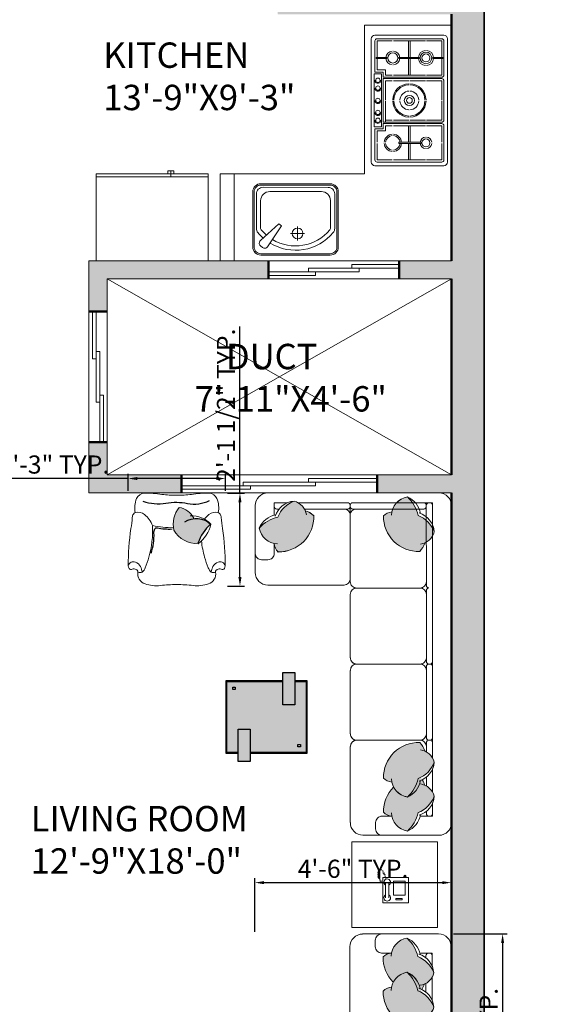
# Model space of a CAD drawing. Units: inches. Extents: x 1734 to 4011, y 1071 to 1891.
# Tile 26 of 27: x 3842 to 3987, y 1313 to 1584. Entities that reach past the tile are written whole.
import ezdxf

# ---------------------------------------------------------------- set-up
doc = ezdxf.new("R2010")
doc.units = ezdxf.units.IN
for name, color, linetype, lineweight in [('A-ANNO-DIMS', 2, 'Continuous', 18), ('A-AREA-IDEN', 3, 'Continuous', 18), ('A-EQPM', 8, 'Continuous', 18), ('A-FLOR-FIXT', 9, 'Continuous', 18), ('A-FURN', 8, 'Continuous', 18), ('A-FURN-PATT', 252, 'Continuous', 13), ('A-GLAZ', 4, 'Continuous', 18), ('A-WALL', 7, 'Continuous', 50), ('A-WALL-PATT', 8, 'Continuous', 13), ('C-PROP', 1, 'Continuous', 35)]:
    doc.layers.add(name, color=color, linetype=linetype, lineweight=lineweight)
doc.layers.add('IFF-FURN-DETAIL', color=250, linetype='Continuous')
doc.layers.add('MOBIL', color=7, linetype='Continuous')
doc.styles.get("Standard").update_dxf_attribs({"font": 'arial.ttf'})
doc.dimstyles.new('ISO-25', dxfattribs={"dimtxt": 5, "dimasz": 2.5, "dimexe": 1.25, "dimexo": 0.625, "dimtad": 1, "dimdec": 1, "dimlunit": 3, "dimtxsty": 'Standard', "dimcen": 2.5, "dimclrt": 1, "dimadec": 0, "dimazin": 0, "dimtfac": 1, "dimtdec": 1, "dimtmove": 0, "dimatfit": 3, "dimfxl": 1, "dimarcsym": 0})

# ---------------------------------------------------------------- blocks, each defined once
blk = doc.blocks.new('STOVE')
for p, q in [((11.85, 19.7), (11.55, 19.7)), ((11.55, 16.92), (11.55, 19.7)), ((11.85, 16.92), (11.85, 19.7)), ((11.85, 16.92), (11.55, 16.92)), ((-11.85, 13.73), (-11.85, 7.62)), ((-11.85, 13.73), (-11.55, 13.73)), ((-11.55, 13.73), (-11.55, 7.62)), ((11.85, 13.23), (11.55, 13.23)), ((11.55, 13.23), (11.55, 7.57)), ((11.85, 13.23), (11.85, 7.57)), ((-11.85, 10.75), (-16.4, 10.75)), ((-11.85, 10.25), (-16.4, 10.25)), ((-7, 10.75), (-11.55, 10.75)), ((-7, 10.25), (-11.55, 10.25)), ((7, 10.75), (11.55, 10.75)), ((7, 10.25), (11.55, 10.25)), ((11.85, 10.75), (16.4, 10.75)), ((11.85, 10.25), (16.4, 10.25)), ((-11.85, 7.62), (-11.55, 7.62)), ((11.85, 7.57), (11.55, 7.57)), ((-7, 3.9), (-8.4, 3.9)), ((-7.8, 3.3), (-7.8, 1)), ((-6.4, 3.3), (-7.8, 3.3)), ((7.3, 2.8), (-7.3, 2.8)), ((-7.3, 2.8), (-7.3, 0.8)), ((-5.4, 3.9), (-6, 3.9)), ((-5.4, 3.9), (-0.15, 3.9)), ((0.15, 3.9), (5.4, 3.9)), ((6.4, 3.3), (7.8, 3.3)), ((7, 3.9), (8.4, 3.9)), ((7.3, 2.8), (7.3, 0.8)), ((7.8, 3.3), (7.8, 1)), ((8.4, 3.9), (8.4, 1.6)), ((11.85, 4.28), (11.55, 4.28)), ((11.55, 4.28), (11.55, 1.3)), ((11.85, 4.28), (11.85, 1.3)), ((7.3, 0.8), (-7.3, 0.8)), ((11.85, 1.3), (11.55, 1.3))]:
    blk.add_line(p, q)
for points in [[(-17, 21), (17, 21, -0.414214), (18, 20), (18, 1, -0.414214), (17, 0), (-17, 0, -0.414214), (-18, 1), (-18, 20, -0.414214)], [(6, 3.3), (-6, 3.3), (-6, 19.4, -0.414214), (-5.4, 20), (5.4, 20, -0.414214), (6, 19.4)]]:
    blk.add_lwpolyline(points, format="xyb", close=True)
for points in [[(-7.8, 1), (-16.4, 1, -0.414214), (-17, 1.6), (-17, 19.4, -0.414214), (-16.4, 20), (-7, 20, -0.414214), (-6.4, 19.4), (-6.4, 3.3)], [(6.4, 19.4, -0.414214), (7, 20), (16.4, 20, -0.414214), (17, 19.4), (17, 1.6, -0.414214), (16.4, 1), (7.8, 1)]]:
    blk.add_lwpolyline(points, format="xyb")
for points in [[(-16.4, 15.22), (-16.4, 19.4), (-11.85, 19.4)], [(-11.55, 19.4), (-7, 19.4), (-7, 15.22)], [(-5.4, 15.22), (-5.4, 19.4), (-0.15, 19.4)], [(0.15, 19.4), (5.4, 19.4), (5.4, 15.22)], [(6.4, 3.3), (6.4, 19.4)], [(7, 15.22), (7, 19.4), (11.55, 19.4)], [(11.85, 19.4), (16.4, 19.4), (16.4, 15.22)], [(-16.4, 6.08), (-16.4, 14.92)], [(-7, 14.92), (-7, 6.08)], [(-5.4, 10.65), (-5.4, 14.92)], [(5.4, 14.92), (5.4, 10.65)], [(7, 6.08), (7, 14.92)], [(16.4, 14.92), (16.4, 6.08)], [(-5.4, 6.08), (-5.4, 10.35)], [(5.4, 10.35), (5.4, 6.08)], [(-11.85, 1.6), (-16.4, 1.6), (-16.4, 5.77)], [(-7, 5.77), (-7, 3.9)], [(-5.4, 3.9), (-5.4, 5.77)], [(5.4, 5.77), (5.4, 3.9)], [(7, 3.9), (7, 5.77)], [(16.4, 5.77), (16.4, 1.6), (11.85, 1.6)], [(-8.4, 3.9), (-8.4, 1.6), (-11.55, 1.6)], [(11.55, 1.6), (8.4, 1.6)]]:
    blk.add_lwpolyline(points)
for centre, radius in [((11.7, 15.07), 1.6), ((-11.7, 15.07), 1.1), ((11.7, 15.07), 1.1), ((0, 10.5), 1.4), ((0, 10.5), 0.8), ((11.7, 5.93), 1.4), ((-5.49, 1.8), 0.6), ((-3.3, 1.8), 0.6), ((0, 1.8), 0.6), ((3.39, 1.8), 0.6), ((5.57, 1.8), 0.6)]:
    blk.add_circle(centre, radius)
for centre, radius, start, end in [((-11.7, 15.07), 1.6, 95.3794, 174.6206), ((-11.7, 15.07), 1.6, 5.3794, 84.6206), ((11.7, 15.07), 2.1, 94.096, 175.904), ((11.7, 15.07), 2.1, 4.096, 85.904), ((-11.7, 15.07), 1.6, 185.3794, 264.6206), ((-11.7, 15.07), 1.6, 275.3794, 354.6206), ((0, 10.5), 4.6, 91.8687, 178.1313), ((0, 10.5), 4.3, 91.9991, 178.0009), ((0, 10.5), 4.6, 1.8687, 88.1313), ((0, 10.5), 4.3, 1.9991, 88.0009), ((11.7, 15.07), 2.1, 184.096, 265.904), ((11.7, 15.07), 2.1, 274.096, 355.904), ((0, 10.5), 2.6, 93.3074, 176.6926), ((0, 10.5), 2.6, 3.3074, 86.6926), ((-11.7, 5.93), 2.4, 93.5833, 176.4167), ((-11.7, 5.93), 2.4, 3.5833, 86.4167), ((0, 10.5), 4.6, 181.8687, 268.1313), ((0, 10.5), 4.3, 181.9991, 268.0009), ((0, 10.5), 2.6, 183.3074, 266.6926), ((0, 10.5), 4.6, 271.8687, 358.1313), ((0, 10.5), 4.3, 271.9991, 358.0009), ((0, 10.5), 2.6, 273.3074, 356.6926), ((-11.7, 5.93), 2.4, 183.5833, 266.4167), ((-11.7, 5.93), 2, 94.3012, 175.6988), ((-11.7, 5.93), 2, 184.3012, 265.6988), ((-11.7, 5.93), 2, 4.3012, 85.6988), ((-11.7, 5.93), 2.4, 273.5833, 356.4167), ((-11.7, 5.93), 2, 274.3012, 355.6988), ((11.7, 5.93), 1.9, 94.5281, 175.4719), ((11.7, 5.93), 1.9, 184.5281, 265.4719), ((11.7, 5.93), 1.9, 4.5281, 85.4719), ((11.7, 5.93), 1.9, 274.5281, 355.4719), ((-5.49, 1.8), 0.846, 89.9979, 270), ((-3.3, 1.8), 0.846, 89.9979, 270), ((0, 1.8), 0.846, 89.9979, 270), ((3.39, 1.8), 0.846, 89.9979, 270), ((5.57, 1.8), 0.846, 89.9979, 270)]:
    blk.add_arc(centre, radius, start, end)
blk = doc.blocks.new('Refrigerator-2 door - 36 in top')
for p, q in [((0, -26.999999), (36, -26.999999)), ((11, -27.999999), (11, -28.999999)), ((12, -26.999999), (12, -28.999999)), ((13, -28.999999), (13, -27.999999)), ((11, -28.999999), (13, -28.999999))]:
    blk.add_line(p, q)
blk.add_lwpolyline([(0, -27.999999), (0, 0), (36, 0), (36, -27.999999)], close=True)
blk = doc.blocks.new('SOFA 1')
at = {"transparency": 33554687}
h = blk.add_hatch(color=256, dxfattribs=at)
h.dxf.hatch_style = 1
h.paths.add_polyline_path([(3723.52, 1308.63, 0.147724), (3717.76, 1305.24, 0.310469), (3722.42, 1300.4), (3722.42, 1300.25, 0.156703), (3723.62, 1297.8, 0.425821), (3734.69, 1309.08, 0.121928), (3732.05, 1310.63, 0.233216), (3728.6, 1313.59, 0.213835)])
h = blk.add_hatch(color=256, dxfattribs=at)
h.dxf.hatch_style = 1
h.paths.add_polyline_path([(3769.65, 1307.6, 0.084911), (3767.15, 1309.12, 0.046133), (3766.46, 1311.13), (3759.18, 1311.13, 0.039409), (3758.92, 1310.24, 0.165523), (3756.31, 1309.02, 0.42585), (3767.59, 1297.95, 0.121928), (3769.15, 1300.58, 0.027403), (3769.65, 1300.83)])
h.paths.add_polyline_path([(3765.34, 1313.08), (3760.4, 1313.08, 0.097704), (3759.18, 1311.13), (3766.46, 1311.13, 0.04873)])
h.paths.add_polyline_path([(3763.76, 1314.88, 0.16488), (3760.4, 1313.08), (3765.34, 1313.08, 0.051917)])
h.paths.add_polyline_path([(3771.6, 1305.17, 0.090388), (3769.65, 1307.6), (3769.65, 1300.83, 0.136035), (3771.6, 1302.77)])
h = blk.add_hatch(color=256, dxfattribs=at)
h.dxf.hatch_style = 1
h.paths.add_polyline_path([(3769.16, 1235.96, 0.122267), (3767.6, 1238.61, 0.425972), (3756.32, 1227.54, 0.165563), (3758.93, 1226.32, 0.309481), (3763.76, 1221.69, 0.002677), (3763.83, 1221.72, 0.146094), (3767.16, 1227.43, 0.212433), (3772.1, 1232.48, 0.235342)])
h = blk.add_hatch(color=256, dxfattribs=at)
h.dxf.hatch_style = 1
h.paths.add_polyline_path([(3769.16, 1225.36, 0.122267), (3767.6, 1228.01, 0.425972), (3756.32, 1216.94, 0.165563), (3758.93, 1215.72, 0.309481), (3763.76, 1211.09, 0.002677), (3763.83, 1211.12, 0.146094), (3767.16, 1216.83, 0.212433), (3772.1, 1221.88, 0.235342)])
for p, q in [((3720.45, 1316.13), (3773.58, 1316.13)), ((3777.51, 1312.19), (3777.51, 1213.72))]:
    blk.add_line(p, q, dxfattribs=at)
for points in [[(3716.51, 1312.2), (3716.51, 1291.44)], [(3722.42, 1313.08), (3722.42, 1309.23), (3722.42, 1313.08), (3726.57, 1313.08)], [(3729.85, 1313.08), (3745.25, 1313.08)], [(3746.01, 1312.3), (3746.01, 1288.55)], [(3768.11, 1313.08), (3746.78, 1313.08)], [(3771.6, 1313.08), (3767.75, 1313.08), (3771.6, 1313.08), (3771.6, 1308.93)], [(3769.66, 1287.39), (3769.65, 1312.3)], [(3771.6, 1313.08), (3771.61, 1233.74)], [(3723.21, 1311.13), (3723.93, 1311.13)], [(3731.82, 1311.13), (3745.25, 1311.13)], [(3746.01, 1310.97), (3746.01, 1311.36)], [(3768.87, 1311.13), (3746.78, 1311.13)], [(3769.65, 1309.43), (3769.65, 1308.71)], [(3746.01, 1288.54), (3746.01, 1308.23)], [(3722.42, 1300.39), (3722.42, 1297.33)], [(3720.45, 1295.38), (3718.48, 1295.38)], [(3720.45, 1287.5), (3744.09, 1287.5)], [(3746.02, 1284.63), (3746.02, 1264.94)], [(3747.99, 1286.6), (3767.69, 1286.6)], [(3769.66, 1263.75), (3769.66, 1285.81)], [(3769.66, 1277.18), (3769.66, 1263.75)], [(3746.02, 1260.99), (3746.02, 1241.3)], [(3747.99, 1262.97), (3767.69, 1262.97)], [(3769.66, 1240.12), (3769.66, 1262.18)], [(3770.43, 1262.97), (3770.82, 1262.97)], [(3747.99, 1239.33), (3767.69, 1239.33)], [(3770.43, 1239.33), (3770.82, 1239.33)], [(3746.02, 1237.36), (3746.02, 1213.74)], [(3769.66, 1235.71), (3769.66, 1238.54)], [(3771.61, 1223.14), (3771.61, 1230.47)], [(3769.66, 1225.11), (3769.66, 1227.82)], [(3767.76, 1215.72), (3771.61, 1215.72), (3771.61, 1219.84), (3771.61, 1215.72)], [(3755.86, 1215.72), (3758.92, 1215.72)], [(3769.66, 1216.5), (3769.66, 1217.22)], [(3753.91, 1211.77), (3753.91, 1213.74)], [(3749.97, 1209.8), (3773.58, 1209.8)]]:
    blk.add_lwpolyline(points, close=True, dxfattribs=at)
for points in [[(3717.76, 1305.24, -0.147724), (3723.52, 1308.63, -0.213355), (3728.59, 1313.59, 0.213355), (3723.52, 1308.63, 0.147724), (3717.76, 1305.24, -0.249545), (3722.86, 1309.34, 0.249545), (3717.75, 1305.25, 0.356779), (3723.4, 1300.28, -0.356779), (3717.76, 1305.24)], [(3728.58, 1313.6, -0.306333), (3732.42, 1309.31, 0.306333), (3728.58, 1313.6, 0.306674), (3722.72, 1308.89, -0.306674), (3728.58, 1313.6)], [(3763.76, 1314.88, -0.147724), (3767.15, 1309.12, -0.213355), (3772.1, 1304.05, 0.213355), (3767.15, 1309.12, 0.147724), (3763.76, 1314.88, -0.249545), (3767.86, 1309.77, 0.249545), (3763.77, 1314.89, 0.356779), (3758.8, 1309.23, -0.356779), (3763.76, 1314.88)], [(3734.69, 1309.08, -0.425972), (3723.62, 1297.8, -0.165552), (3722.4, 1300.4, 0.165552), (3723.62, 1297.79, 0.425972), (3734.69, 1309.07, 0.121514), (3732.07, 1310.63, -0.121514), (3734.69, 1309.08)], [(3767.6, 1297.95, -0.425972), (3756.31, 1309.01, -0.165552), (3758.92, 1310.24, 0.165552), (3756.31, 1309.02, 0.425972), (3767.59, 1297.95, 0.121514), (3769.14, 1300.57, -0.121514), (3767.6, 1297.95)], [(3772.11, 1304.06, -0.306333), (3767.83, 1300.22, 0.306333), (3772.11, 1304.06, 0.306674), (3767.4, 1309.91, -0.306674), (3772.11, 1304.06)], [(3770.44, 1286.63, -0.414214), (3769.66, 1287.4, 0.414214), (3770.44, 1286.63, 0.414214), (3769.66, 1285.83, -0.414214), (3770.44, 1286.63)], [(3748.01, 1262.99, -0.414214), (3746.05, 1264.95, 0.414214), (3748.01, 1262.97, 0.414213), (3746.05, 1261.01, -0.414213), (3748.01, 1262.99)], [(3770.44, 1262.99, -0.414214), (3769.66, 1263.77, 0.414214), (3770.44, 1262.99, 0.414214), (3769.66, 1262.19, -0.414214), (3770.44, 1262.99)], [(3770.83, 1262.97, -0.414214), (3771.61, 1262.19, 0.414214), (3770.83, 1262.99, 0.414214), (3771.61, 1263.77, -0.414214), (3770.83, 1262.97)], [(3748.01, 1239.35, -0.414214), (3746.05, 1241.31, 0.414214), (3748.01, 1239.33, 0.414213), (3746.05, 1237.37, -0.414213), (3748.01, 1239.35)], [(3767.7, 1239.33, -0.414214), (3769.66, 1237.37, 0.414214), (3767.7, 1239.35, 0.414214), (3769.66, 1241.31, -0.414214), (3767.7, 1239.33)], [(3770.44, 1239.35, -0.414214), (3769.66, 1240.13, 0.414214), (3770.44, 1239.33, 0.414214), (3769.66, 1238.55, -0.414214), (3770.44, 1239.35)], [(3770.83, 1239.33, -0.414214), (3771.61, 1238.55, 0.414214), (3770.83, 1239.35, 0.414214), (3771.61, 1240.13, -0.414214), (3770.83, 1239.33)], [(3756.32, 1227.54, -0.425972), (3767.6, 1238.61, -0.121514), (3769.16, 1235.98, 0.121514), (3767.6, 1238.61, 0.425972), (3756.32, 1227.54, 0.165552), (3758.93, 1226.32, -0.165552), (3756.32, 1227.54)], [(3772.1, 1232.5, -0.306674), (3767.41, 1226.64, 0.306674), (3772.1, 1232.5, 0.306333), (3767.84, 1236.34, -0.306333), (3772.1, 1232.5)], [(3763.78, 1221.67, 0.249545), (3767.87, 1226.78, -0.249545), (3763.76, 1221.69, -0.356779), (3758.81, 1227.32, 0.356779), (3763.77, 1221.68, 0.147724), (3767.16, 1227.43, 0.213355), (3772.11, 1232.51, -0.213355), (3767.16, 1227.43, -0.147724), (3763.78, 1221.67)], [(3756.32, 1216.94, -0.200233), (3759.49, 1224.76, 0.200233), (3756.32, 1216.94, 0.165552), (3758.93, 1215.72, -0.165552), (3756.32, 1216.94)], [(3772.1, 1221.9, -0.306674), (3767.41, 1216.04, 0.306674), (3772.1, 1221.9, -0.213355), (3767.16, 1216.83, -0.147724), (3763.77, 1211.08, 0.147724), (3767.15, 1216.83, 0.213355), (3772.1, 1221.9)], [(3763.76, 1211.09, -0.356779), (3758.81, 1216.72, 0.356779), (3763.76, 1211.09, 0.249545), (3767.87, 1216.18, -0.249545), (3763.76, 1211.09)]]:
    blk.add_lwpolyline(points, format="xyb", dxfattribs=at)
for points in [[(3770.43, 1313.08, 0.414214), (3769.65, 1312.3, -0.414214)], [(3771.6, 1312.3, 0.414214), (3770.82, 1313.08, -0.414214)], [(3722.42, 1311.91, 0.414214), (3723.2, 1311.13, -0.414214)], [(3716.51, 1297.34, 0.414214), (3718.47, 1295.38, -0.414214)], [(3720.44, 1295.38, 0.414214), (3722.4, 1297.34, -0.414214)], [(3716.51, 1291.45, 0.414212), (3720.44, 1287.52, -0.414212)], [(3746.03, 1288.56, 0.414214), (3747.99, 1286.6, 0.414213), (3746.03, 1284.64, -0.414213), (3747.99, 1286.6, -0.414214)], [(3769.66, 1284.64, 0.414214), (3767.7, 1286.6, 0.414214), (3769.66, 1288.56, -0.414214), (3767.7, 1286.6, -0.414214)], [(3769.66, 1261.01, 0.414214), (3767.7, 1262.97, 0.414214), (3769.66, 1264.93, -0.414214), (3767.7, 1262.97, -0.414214)], [(3769.16, 1225.36, 0.071861), (3768.39, 1227.01, -0.071861)], [(3772.13, 1221.9, 0.306333), (3767.84, 1225.74, -0.306333)], [(3755.87, 1215.72, 0.414214), (3753.91, 1213.76, -0.414214)], [(3769.66, 1216.52, 0.414214), (3770.44, 1215.74, -0.414214)], [(3770.83, 1215.74, 0.414214), (3771.61, 1216.52, -0.414214)], [(3746.05, 1213.76, 0.414212), (3749.98, 1209.82, -0.414212)], [(3755.87, 1209.8, -0.414214), (3753.91, 1211.76, 0.414214)]]:
    blk.add_lwpolyline(points, format="xyb", close=True, dxfattribs=at)
for centre, radius, start, end in [((3720.44, 1312.2), 3.93, 90.0002, 179.9998), ((3720.44, 1312.19), 3.94, 89.9158, 179.9154), ((3773.58, 1312.2), 3.93, 0.0002, 89.9998), ((3773.57, 1312.19), 3.94, 359.9158, 89.9154), ((3745.22, 1312.29), 0.789, 0.8425, 90.8425), ((3746.8, 1312.29), 0.789, 89.1575, 179.1575), ((3768.87, 1312.3), 0.777, 360, 90), ((3744.09, 1309.21), 1.92, 358.766, 90.5111), ((3745.24, 1311.91), 0.777, 270, 0), ((3745.24, 1311.91), 0.777, 270, 0), ((3746.79, 1311.91), 0.777, 180, 270), ((3746.79, 1311.91), 0.777, 180, 270), ((3747.93, 1309.21), 1.92, 89.4889, 181.234), ((3768.87, 1311.91), 0.777, 270, 0), ((3744.08, 1289.48), 1.96, 270, 360), ((3744.08, 1289.48), 1.96, 270, 360), ((3773.58, 1213.73), 3.93, 270.0002, 359.9998), ((3773.59, 1213.73), 3.93, 269.9156, 359.9152)]:
    blk.add_arc(centre, radius, start, end, dxfattribs=at)
blk = doc.blocks.new('Mesa de centro Cantria feeling')
at = {"layer": 'MOBIL', "ltscale": 0.2}
h = blk.add_hatch(color=256, dxfattribs=at)
h.set_gradient(color1=(74, 55, 38), color2=(104, 77, 54), one_color=1, tint=0.31, name='CYLINDER')
h.paths.add_polyline_path([(-0.85, -0.3), (-0.7, -0.3), (-0.7, 0.1), (-0.85, 0.1)])
h = blk.add_hatch(color=256, dxfattribs=at)
h.set_gradient(color1=(221, 221, 223), one_color=1, tint=1)
h.paths.add_polyline_path([(-0.15, -0.6), (-0.15, -0.89), (-0.01, -0.89), (-0.01, -0.01), (-0.7, -0.01), (-0.7, -0.3), (-0.85, -0.3), (-0.85, -0.01), (-0.99, -0.01), (-0.99, -0.89), (-0.3, -0.89), (-0.3, -0.6)])
h.paths.add_polyline_path([(-0.112, -0.112), (-0.112, -0.082), (-0.082, -0.082), (-0.082, -0.112)], flags=16)
h.paths.add_polyline_path([(-0.888, -0.788), (-0.888, -0.818), (-0.918, -0.818), (-0.918, -0.788)], flags=16)
h = blk.add_hatch(color=256, dxfattribs=at)
h.set_gradient(color1=(74, 55, 38), color2=(104, 77, 54), one_color=1, tint=0.31, name='CYLINDER')
h.paths.add_polyline_path([(-0.15, -0.6), (-0.3, -0.6), (-0.3, -1), (-0.15, -1)])
for points in [[(-0.85, 0), (-1, 0), (-1, -0.9), (-0.3, -0.9)], [(-0.15, -0.9), (0, -0.9), (0, 0), (-0.7, 0)], [(-0.85, -0.01), (-0.99, -0.01), (-0.99, -0.89), (-0.3, -0.89)], [(-0.15, -0.89), (-0.01, -0.89), (-0.01, -0.01), (-0.7, -0.01)]]:
    blk.add_lwpolyline(points, dxfattribs=at)
for points in [[(-0.85, -0.3), (-0.7, -0.3), (-0.7, 0.1), (-0.85, 0.1)], [(-0.082, -0.082), (-0.112, -0.082), (-0.112, -0.112), (-0.082, -0.112)], [(-0.15, -0.6), (-0.3, -0.6), (-0.3, -1), (-0.15, -1)], [(-0.918, -0.818), (-0.888, -0.818), (-0.888, -0.788), (-0.918, -0.788)]]:
    blk.add_lwpolyline(points, close=True, dxfattribs=at)
blk = doc.blocks.new('PILLOW-1')
at = {"color": 0}
blk.add_lwpolyline([(198, -165.3, -0.232884), (126.3, -346, -0.184752), (-44.3, -233.7, -0.286563), (74.8, -22, -0.237978), (272.6, -68.2, -0.243587), (179.4, -195.4, 4.263709)], format="xyb", dxfattribs=at)
at = {"layer": 'IFF-FURN-DETAIL'}
blk.add_lwpolyline([(147.6, -117.6, -0.343333), (126.5, -342.2, 0.126408), (-39.5, -232.6, -5.969376)], format="xyb", dxfattribs=at)
blk = doc.blocks.new('CLNG90')
for points in [[(689.4, 369.7, 0.157831), (676.6, 385.2, 0.121013), (646.4, 395.4, -0.017334), (546.8, 407.4, 0.041496), (215.3, 431.2, 0.153531), (191.4, 423.4, 0.382906), (185.1, 395.3, -0.284047), (183.7, 360.8, 0.011997), (177.2, 350.7, -0.370479), (159.9, 345, 0.380647), (56.2, 282, 0.117468), (40.6, 145.8, -0.027775), (50, 0, -8.773898)], [(159.9, 345, 0.22481), (159.8, 306.3, 0.055398), (209.2, 321.6, 0.180116), (248.9, 368.2, 0.194833), (247.6, 405.4, 0.242377), (215.3, 431.2, 1.52074)], [(159.9, 345, 0.22481), (159.8, 306.3, 0.055398), (209.2, 321.6, 0.180116), (248.9, 368.2, 0.194833), (247.6, 405.4, 0.242377), (215.3, 431.2, 1.52074)], [(689.4, 369.7, -0.235486), (671.3, 286, -0.134038), (573.9, 215.1, -0.079303), (292.9, 247.8, -0.027048), (199.2, 279.7, -0.106276), (159.8, 306.3, -1.699)], [(689.4, 369.7, -0.235486), (671.3, 286, -0.134038), (573.9, 215.1, -0.079303), (292.9, 247.8, -0.027048), (199.2, 279.7, -0.106276), (159.8, 306.3, -1.699)], [(689.4, 369.7, -0.146607), (813.9, 357.3, -0.305296), (861.7, 285.6, -0.042137), (851.9, 131.4, 0.040285), (843.1, 0, 3.952121)], [(573.9, 215.1, 0.061244), (555.6, 29, 3.376255)], [(573.9, 215.1, 0.061244), (555.6, 29, 3.376255)], [(689.4, -369.7, -0.157831), (676.6, -385.2, -0.121013), (646.4, -395.4, 0.017334), (546.8, -407.4, -0.041496), (215.3, -431.2, -0.153531), (191.4, -423.4, -0.382906), (185.1, -395.3, 0.284047), (183.7, -360.8, -0.011997), (177.2, -350.7, 0.370479), (159.9, -345, -0.380647), (56.2, -282, -0.117468), (40.6, -145.8, 0.027775), (50, 0, 8.773898)], [(689.4, -369.7, 0.146607), (813.9, -357.3, 0.305296), (861.7, -285.6, 0.042137), (851.9, -131.4, -0.040285), (843.1, 0, -3.952121)], [(437.4, -219.7, 0.041086), (292.9, -247.8, 0.027048), (199.2, -279.7, 0.106276), (159.8, -306.3, 1.699)], [(437.4, -219.7, 0.041086), (292.9, -247.8, 0.027048), (199.2, -279.7, 0.106276), (159.8, -306.3, 1.699)], [(689.4, -369.7, 0.235486), (671.3, -286, 0.060693), (631.8, -247.3, 0.001296)], [(689.4, -369.7, 0.235486), (671.3, -286, 0.060693), (631.8, -247.3, 0.001296)], [(159.9, -345, -0.22481), (159.8, -306.3, -0.055398), (209.2, -321.6, -0.180116), (248.9, -368.2, -0.194833), (247.6, -405.4, -0.242377), (215.3, -431.2, -1.52074)], [(159.9, -345, -0.22481), (159.8, -306.3, -0.055398), (209.2, -321.6, -0.180116), (248.9, -368.2, -0.194833), (247.6, -405.4, -0.242377), (215.3, -431.2, -1.52074)]]:
    blk.add_lwpolyline(points, format="xyb")
at = {"layer": 'IFF-FURN-DETAIL'}
for points in [[(790.6, 301.1, 0.124986), (773.9, 95.7, -0.091334), (771.1, -94.9, 0.164688), (796.9, -292.4, 1.068868)], [(790.6, 301.1, 0.124986), (773.9, 95.7, -0.091334), (771.1, -94.9, 0.164688), (796.9, -292.4, 1.068868)], [(328.2, 228.3, 0.109125), (508.5, 203.4, -0.16587), (546, 193.9, -0.314359), (554.8, 172.3, 0.072017), (544.2, 42.1, 4.351186)], [(328.2, 228.3, 0.109125), (508.5, 203.4, -0.16587), (546, 193.9, -0.314359), (554.8, 172.3, 0.072017), (544.2, 42.1, 4.351186)]]:
    blk.add_lwpolyline(points, format="xyb", dxfattribs=at)
at = {"xscale": 1.016, "yscale": 1.016, "zscale": 1.016}
blk.add_blockref('PILLOW-1', (458.1, 47.3), dxfattribs=at)
blk.add_blockref('PILLOW-1', (458.1, 47.3), dxfattribs=at)
blk = doc.blocks.new('*D85')
at = {"layer": 'A-ANNO-DIMS', "color": 0, "lineweight": -2, "transparency": 16777216}
for p, q in [((3961.35, 1332.21), (3976.13, 1332.21)), ((3974.88, 1329.71), (3974.88, 1240.32)), ((3961.35, 1237.82), (3976.13, 1237.82))]:
    blk.add_line(p, q, dxfattribs=at)
at = {"layer": 'A-ANNO-DIMS', "color": 0, "transparency": 16777216}
for points in [[(3974.47, 1329.71), (3975.3, 1329.71), (3974.88, 1332.21)], [(3974.47, 1240.32), (3975.3, 1240.32), (3974.88, 1237.82)]]:
    blk.add_solid(points, dxfattribs=at)
at = {"layer": 'Defpoints', "color": 0, "transparency": 16777216}
for p in [(3960.72, 1332.21), (3960.72, 1237.82), (3974.88, 1237.82)]:
    blk.add_point(p, dxfattribs=at)
at = {"layer": 'A-ANNO-DIMS', "color": 1, "transparency": 16777216, "insert": (3971.67, 1285.01), "char_height": 5, "attachment_point": 5, "rotation": 90}
blk.add_mtext('SOFA 7\'-10 1/2" TYP.', dxfattribs=at)
blk = doc.blocks.new('*D86')
at = {"layer": 'A-ANNO-DIMS', "color": 0, "lineweight": -2, "transparency": 16777216}
for p, q in [((3906.57, 1332.83), (3906.57, 1347.62)), ((3960.72, 1332.83), (3960.72, 1347.62)), ((3909.07, 1346.37), (3958.22, 1346.37))]:
    blk.add_line(p, q, dxfattribs=at)
at = {"layer": 'A-ANNO-DIMS', "color": 0, "transparency": 16777216}
for points in [[(3909.07, 1346.78), (3909.07, 1345.95), (3906.57, 1346.37)], [(3958.22, 1346.78), (3958.22, 1345.95), (3960.72, 1346.37)]]:
    blk.add_solid(points, dxfattribs=at)
at = {"layer": 'Defpoints', "color": 0, "transparency": 16777216}
for p in [(3960.72, 1346.37), (3906.57, 1332.21), (3960.72, 1332.21)]:
    blk.add_point(p, dxfattribs=at)
at = {"layer": 'A-ANNO-DIMS', "color": 1, "transparency": 16777216, "insert": (3933.65, 1349.54), "char_height": 5, "attachment_point": 5}
blk.add_mtext('4\'-6" TYP.', dxfattribs=at)
blk = doc.blocks.new('*D87')
at = {"layer": 'A-ANNO-DIMS', "color": 0, "lineweight": -2, "transparency": 16777216}
for p, q in [((3871.63, 1454.4), (3871.63, 1459.05)), ((3898.44, 1454.4), (3898.44, 1459.05)), ((3871.63, 1457.8), (3797.91, 1457.8)), ((3895.94, 1457.8), (3874.13, 1457.8))]:
    blk.add_line(p, q, dxfattribs=at)
at = {"layer": 'A-ANNO-DIMS', "color": 0, "transparency": 16777216}
for points in [[(3874.13, 1458.22), (3874.13, 1457.38), (3871.63, 1457.8)], [(3895.94, 1458.22), (3895.94, 1457.38), (3898.44, 1457.8)]]:
    blk.add_solid(points, dxfattribs=at)
at = {"layer": 'Defpoints', "color": 0, "transparency": 16777216}
for p in [(3871.63, 1457.8), (3871.63, 1453.78), (3898.44, 1453.78)]:
    blk.add_point(p, dxfattribs=at)
at = {"layer": 'A-ANNO-DIMS', "color": 1, "transparency": 16777216, "insert": (3833.52, 1461.01), "char_height": 5, "attachment_point": 5}
blk.add_mtext('ARMCHAIR 2\'-3" TYP.', dxfattribs=at)
blk = doc.blocks.new('*D88')
at = {"layer": 'A-ANNO-DIMS', "color": 0, "lineweight": -2, "transparency": 16777216}
for p, q in [((3902.46, 1453.78), (3902.46, 1499.74)), ((3899.06, 1453.78), (3903.71, 1453.78)), ((3902.46, 1430.62), (3902.46, 1451.28)), ((3899.06, 1428.12), (3903.71, 1428.12))]:
    blk.add_line(p, q, dxfattribs=at)
at = {"layer": 'A-ANNO-DIMS', "color": 0, "transparency": 16777216}
for points in [[(3902.04, 1451.28), (3902.88, 1451.28), (3902.46, 1453.78)], [(3902.04, 1430.62), (3902.88, 1430.62), (3902.46, 1428.12)]]:
    blk.add_solid(points, dxfattribs=at)
at = {"layer": 'Defpoints', "color": 0, "transparency": 16777216}
for p in [(3898.44, 1453.78), (3902.46, 1453.78), (3898.44, 1428.12)]:
    blk.add_point(p, dxfattribs=at)
at = {"layer": 'A-ANNO-DIMS', "color": 1, "transparency": 16777216, "insert": (3899.25, 1478.01), "char_height": 5, "attachment_point": 5, "rotation": 90}
blk.add_mtext('2\'-1 1/2" TYP.', dxfattribs=at)

msp = doc.modelspace()

# ---------------------------------------------------------------- hatches: boundary and pattern name
at = {"layer": 'A-FURN-PATT'}
h = msp.add_hatch(dxfattribs=at)
h.set_pattern_fill('ANSI32', color=256)
h.set_pattern_definition([(45, (598.983, -12.241), (-6.735192, 6.735192), []), (45, (603.473, -12.241), (-6.735192, 6.735192), [])])
h.paths.add_polyline_path([(3723.83, 1453.82), (3663.83, 1453.82), (3663.83, 1435.82), (3723.83, 1435.82)])
h.paths.add_polyline_path([(3667.71, 1440.04), (3717.17, 1440.04), (3717.17, 1450.34), (3667.71, 1450.34)], flags=24)
h.paths.add_polyline_path([(3882.46, 1633.93), (3882.46, 1688.64), (3856.34, 1688.64), (3856.34, 1633.93)], flags=9)
h.paths.add_polyline_path([(3912.44, 1633.93), (3912.44, 1688.64), (3886.32, 1688.64), (3886.32, 1633.93)], flags=9)
h.paths.add_polyline_path([(3849.42, 1795.58), (3903.83, 1795.58), (3903.83, 1821.7), (3849.42, 1821.7)], flags=9)
h.paths.add_polyline_path([(3821.75, 1770.76), (3864.43, 1770.76), (3864.43, 1779), (3821.75, 1779)], flags=9)
h.paths.add_polyline_path([(3824.93, 1134.29), (3837.52, 1134.29), (3837.52, 1144.59), (3824.93, 1144.59)], flags=9)
h.paths.add_polyline_path([(3824.92, 1203.29), (3837.13, 1203.29), (3837.13, 1213.59), (3824.92, 1213.59)], flags=9)
h.paths.add_polyline_path([(3649.53, 1633.93), (3649.53, 1688.64), (3623.41, 1688.64), (3623.41, 1633.93)], flags=9)
h.paths.add_polyline_path([(3861.96, 1555.4), (3916.37, 1555.4), (3916.37, 1581.52), (3861.96, 1581.52)], flags=9)
h.paths.add_polyline_path([(3920.06, 1601.91), (3940.42, 1601.91), (3940.42, 1612.21), (3920.06, 1612.21)], flags=9)
h.paths.add_polyline_path([(3879.75, 1638.04), (3929.21, 1638.04), (3929.21, 1648.34), (3879.75, 1648.34)], flags=9)
h.paths.add_polyline_path([(3861.7, 1695.43), (3921.55, 1695.43), (3921.55, 1721.55), (3861.7, 1721.55)], flags=9)
h.paths.add_polyline_path([(3738.69, 1778.27), (3787.65, 1778.27), (3787.65, 1804.39), (3738.69, 1804.39)], flags=9)
h.paths.add_polyline_path([(3649.33, 1778.26), (3698.3, 1778.26), (3698.3, 1804.38), (3649.33, 1804.38)], flags=9)
h.paths.add_polyline_path([(3687.88, 1211.9), (3747.72, 1211.9), (3747.72, 1238.02), (3687.88, 1238.02)], flags=9)
h.paths.add_polyline_path([(3782.95, 1496.7), (3837.36, 1496.7), (3837.36, 1522.82), (3782.95, 1522.82)], flags=9)
h.paths.add_polyline_path([(3862.83, 1344.86), (3931.88, 1344.86), (3931.88, 1370.98), (3862.83, 1370.98)], flags=9)
h.paths.add_polyline_path([(3887.8, 1472.31), (3942.21, 1472.31), (3942.21, 1498.43), (3887.8, 1498.43)], flags=9)
h.paths.add_polyline_path([(3707.14, 1647.71), (3772.42, 1647.71), (3772.42, 1673.83), (3707.14, 1673.83)], flags=9)
h = msp.add_hatch(color=256, dxfattribs=at)
h.dxf.hatch_style = 1
h.paths.add_polyline_path([(3890.84, 1439.83, -0.129718), (3894.34, 1445.21, 0.218011), (3889.78, 1446.76, 0.250405), (3885.72, 1449.82, 0.237978), (3884.26, 1443.59, 0.283254)])
at = {"layer": 'A-WALL-PATT'}
h = msp.add_hatch(color=256, dxfattribs=at)
h.dxf.hatch_style = 1
h.paths.add_polyline_path([(3969.83, 1831.82), (3618.83, 1831.82), (3618.83, 1745.82), (3627.39, 1745.82), (3627.39, 1750.82), (3623.83, 1750.82), (3623.83, 1822.82), (3710.83, 1822.82), (3710.83, 1780.82), (3715.83, 1780.82), (3715.83, 1822.82), (3802.83, 1822.82), (3802.83, 1750.82), (3750.83, 1750.82), (3750.83, 1745.82), (3802.83, 1745.82), (3802.83, 1604.82), (3807.83, 1604.82), (3807.83, 1628.82), (3811.83, 1628.82), (3811.83, 1633.82), (3807.83, 1633.82), (3807.83, 1777.82), (3813.86, 1777.82), (3813.86, 1786.82), (3807.83, 1786.82), (3807.83, 1826.82), (3960.83, 1826.82), (3960.83, 1786.82), (3942.83, 1786.82), (3942.83, 1777.82), (3960.83, 1777.82), (3960.83, 1633.82), (3847.83, 1633.82), (3847.83, 1628.82), (3960.83, 1628.82), (3960.83, 1588.82), (3912.83, 1588.82), (3912.83, 1585.82), (3960.83, 1585.82), (3960.83, 1517.82), (3946.33, 1517.82), (3946.33, 1512.82), (3960.83, 1512.82), (3960.83, 1458.82), (3940.33, 1458.82), (3940.33, 1453.82), (3969.83, 1453.82)])
h.paths.add_polyline_path([(3969.83, 1453.82), (3960.83, 1453.82), (3960.83, 1237.82), (3866.83, 1237.82), (3866.83, 1228.82), (3960.83, 1228.82), (3960.83, 1120.82), (3785.83, 1120.82), (3785.83, 1111.82), (3969.83, 1111.82)])
h = msp.add_hatch(color=256, dxfattribs=at)
h.dxf.hatch_style = 1
h.paths.add_polyline_path([(3860.83, 1503.82), (3865.83, 1503.82), (3865.83, 1512.82), (3910.33, 1512.82), (3910.33, 1517.82), (3860.83, 1517.82)])
h.paths.add_polyline_path([(3860.83, 1453.82), (3886.33, 1453.82), (3886.33, 1458.82), (3865.83, 1458.82), (3865.83, 1467.82), (3860.83, 1467.82)])

# ---------------------------------------------------------------- linework, layer by layer
at = {"layer": 'A-FLOR-FIXT'}
msp.add_circle((3918.34, 1525.37), 1.5, dxfattribs=at)
at = {"layer": 'A-FURN'}
for p, q in [((3936.83, 1582.82), (3936.83, 1541.82)), ((3936.83, 1582.82), (3960.83, 1582.82)), ((3897, 1541.82), (3936.83, 1541.82)), ((3897, 1517.82), (3897, 1541.82)), ((3900.83, 1541.82), (3900.83, 1517.82)), ((3860.83, 1517.82), (3960.83, 1517.82)), ((3860.83, 1517.82), (3860.83, 1453.82)), ((3865.83, 1512.82), (3960.83, 1512.82)), ((3865.83, 1512.82), (3865.83, 1458.82)), ((3865.83, 1512.82), (3960.83, 1458.82)), ((3865.83, 1458.82), (3960.83, 1512.82)), ((3865.83, 1458.82), (3960.83, 1458.82)), ((3860.83, 1453.82), (3960.83, 1453.82))]:
    msp.add_line(p, q, dxfattribs=at)
for points in [[(3908.23, 1539.09, 0.414214), (3905.99, 1536.86), (3906.01, 1521.64, 0.414214), (3908.22, 1519.4), (3927.37, 1519.42, 0.414214), (3929.58, 1521.62), (3929.58, 1536.86, 0.414214), (3927.35, 1539.09), (3908.23, 1539.09)], [(3908.23, 1538.72, 0.414214), (3906.39, 1536.86), (3906.39, 1521.64, 0.414214), (3908.22, 1519.79), (3927.37, 1519.79, 0.414214), (3929.19, 1521.62), (3929.19, 1536.86, 0.414214), (3927.35, 1538.7), (3908.23, 1538.72)], [(3910.75, 1522.74, 0.371519), (3928.18, 1525.6, 0.175764), (3928.58, 1526.77), (3928.61, 1536.27, 0.414214), (3926.75, 1538.09), (3908.83, 1538.12, 0.414214), (3906.99, 1536.26), (3906.99, 1526.77, 0.175764), (3907.42, 1525.6, 0.038632), (3908.87, 1524.12)], [(3911.4, 1523.73, 0.370401), (3927.27, 1526.36, 0.175764), (3927.4, 1526.77), (3927.4, 1534.42, 0.414214), (3924.9, 1536.91), (3910.69, 1536.91, 0.414214), (3908.17, 1534.41), (3908.17, 1526.77, 0.175764), (3908.33, 1526.36, 0.038512), (3909.77, 1524.91)]]:
    msp.add_lwpolyline(points, format="xyb", dxfattribs=at)
for points in [[(3908.1, 1522), (3908.68, 1521.51, 0.463205), (3910.07, 1521.72), (3913.9, 1527.45), (3913.2, 1528.05), (3908.12, 1523.41, 0.4637)], [(3943.5, 1345.7, 3.938511), (3942.63, 1345.7, -3.938511)], [(3942.63, 1342.97, 3.938511), (3943.5, 1342.97, -3.938511)]]:
    msp.add_lwpolyline(points, format="xyb", close=True, dxfattribs=at)
for points in [[(3918.33, 1523.41), (3918.33, 1527.31)], [(3920.28, 1525.36), (3916.38, 1525.36)], [(3956.95, 1357.63), (3956.95, 1334.01), (3933.33, 1334.01), (3933.33, 1357.63)]]:
    msp.add_lwpolyline(points, dxfattribs=at)
for points in [[(3933.33, 1334.01), (3933.33, 1357.63), (3956.95, 1357.63), (3956.95, 1334.01)], [(3940.52, 1349.53), (3941.04, 1349.37)], [(3940.69, 1349.88), (3941.22, 1349.72)], [(3941.1, 1350.13), (3941.62, 1349.95)], [(3941.57, 1349.72), (3942.08, 1349.53)], [(3940.87, 1347.12), (3941.38, 1346.93)], [(3941.82, 1347.81), (3948.92, 1347.81), (3948.92, 1340.81), (3941.82, 1340.81)], [(3948.92, 1347.81), (3948.92, 1340.81), (3941.82, 1340.81), (3941.82, 1347.81)], [(3947.99, 1342.94), (3944.75, 1342.94), (3944.75, 1346.75), (3947.99, 1346.75)], [(3944.75, 1342.94), (3944.75, 1346.75), (3947.99, 1346.75), (3947.99, 1342.94)], [(3942.61, 1346.49), (3942.61, 1342.15)], [(3943.47, 1346.49), (3943.47, 1342.15)], [(3947.18, 1341.99), (3947.18, 1341.6), (3945.44, 1341.6), (3945.44, 1341.99)], [(3945.44, 1341.99), (3947.18, 1341.99), (3947.18, 1341.6), (3945.44, 1341.6)]]:
    msp.add_lwpolyline(points, close=True, dxfattribs=at)
at = {"layer": 'A-GLAZ'}
for p, q in [((3921.33, 1514.82), (3921.33, 1515.82)), ((3921.33, 1515.82), (3946.33, 1515.82)), ((3933.33, 1515.82), (3933.33, 1516.82)), ((3933.33, 1516.82), (3946.33, 1516.82)), ((3935.33, 1514.82), (3935.33, 1515.82)), ((3910.33, 1514.82), (3935.33, 1514.82)), ((3910.33, 1513.82), (3923.33, 1513.82)), ((3923.33, 1513.82), (3923.33, 1514.82)), ((3861.83, 1490.82), (3861.83, 1503.82)), ((3862.83, 1478.82), (3862.83, 1503.82)), ((3862.83, 1490.82), (3861.83, 1490.82)), ((3863.83, 1492.82), (3862.83, 1492.82)), ((3863.83, 1467.82), (3863.83, 1492.82)), ((3864.83, 1480.82), (3863.83, 1480.82)), ((3864.83, 1467.82), (3864.83, 1480.82)), ((3863.83, 1478.82), (3862.83, 1478.82)), ((3886.33, 1455.82), (3923.33, 1455.82)), ((3903.33, 1456.82), (3903.33, 1455.82)), ((3903.33, 1456.82), (3940.33, 1456.82)), ((3905.33, 1455.82), (3905.33, 1454.82)), ((3921.33, 1457.82), (3921.33, 1456.82)), ((3921.33, 1457.82), (3940.33, 1457.82)), ((3923.33, 1456.82), (3923.33, 1455.82)), ((3886.33, 1454.82), (3905.33, 1454.82))]:
    msp.add_line(p, q, dxfattribs=at)
for points in [[(3941.73, 1349.37), (3942.24, 1349.18)], [(3940.34, 1349.18), (3940.87, 1349.02)], [(3940.34, 1348.83), (3940.87, 1348.67)], [(3940.34, 1348.49), (3940.87, 1348.32)], [(3940.34, 1348.14), (3940.87, 1347.98)], [(3940.52, 1347.81), (3941.04, 1347.63)], [(3940.69, 1347.47), (3941.22, 1347.28)], [(3941.04, 1346.77), (3941.57, 1346.58)], [(3941.89, 1349.02), (3942.43, 1348.83)], [(3942.08, 1348.67), (3942.59, 1348.49)], [(3942.43, 1348.32), (3942.73, 1347.33)], [(3941.22, 1346.42), (3941.73, 1346.24)]]:
    msp.add_lwpolyline(points, close=True, dxfattribs=at)
at = {"layer": 'A-WALL'}
for p, q in [((3960.83, 1585.82), (3960.83, 1517.82)), ((3910.33, 1512.82), (3910.33, 1517.82)), ((3946.33, 1512.82), (3946.33, 1517.82)), ((3960.83, 1512.82), (3960.83, 1458.82)), ((3865.83, 1503.82), (3860.83, 1503.82)), ((3865.83, 1467.82), (3860.83, 1467.82)), ((3886.33, 1458.82), (3886.33, 1453.82)), ((3940.33, 1458.82), (3940.33, 1453.82)), ((3960.83, 1453.82), (3960.83, 1237.82))]:
    msp.add_line(p, q, dxfattribs=at)
at = {"layer": 'C-PROP'}
msp.add_lwpolyline([(3785.83, 1111.82), (3609.83, 1111.82), (3609.83, 1831.82), (3969.83, 1831.82), (3969.83, 1111.82), (3785.83, 1111.82)], dxfattribs=at)

# ---------------------------------------------------------------- block references
at = {"layer": 'A-EQPM', "xscale": -1, "rotation": 270}
msp.add_blockref('STOVE', (3938.68, 1562.06), dxfattribs=at)
at = {"layer": 'A-EQPM', "xscale": 0.8569942030484906, "yscale": 0.8569942030484906, "zscale": 0.8569942030484906, "rotation": 180}
msp.add_blockref('Refrigerator-2 door - 36 in top', (3893.68, 1517.82), dxfattribs=at)
at = {"layer": 'A-FURN'}
for name, p, xscale, yscale, zscale, rotation in [('CLNG90', (3885.03, 1427.03), 0.031001591544, 0.031001591544, 0.031001591544, 90), ('Mesa de centro Cantria feeling', (3920.94, 1382), -22.3138190187957, 22.3138190187957, 22.3138190187957, 180), ('SOFA 1', (607.6, 2406.09), -0.887653230693335, 0.887653230693335, 0.887653230693335, 180)]:
    msp.add_blockref(name, p, dxfattribs=dict(at, xscale=xscale, yscale=yscale, zscale=zscale, rotation=rotation))
at = {"layer": 'A-FURN', "xscale": 0.887653230693335, "yscale": 0.887653230693335, "zscale": 0.887653230693335}
msp.add_blockref('SOFA 1', (607.7, 285.55), dxfattribs=at)

# ---------------------------------------------------------------- texts
at = {"layer": 'A-AREA-IDEN', "char_height": 7, "attachment_point": 1}
for s, insert in [('KITCHEN\\P13\'-9"X9\'-3"', (3864.78, 1578.04)), ('    DUCT\\P7\'-11"X4\'-6"', (3890.01, 1494.94)), ('LIVING ROOM\\P12\'-9"X18\'-0"', (3844.76, 1367.5))]:
    msp.add_mtext_dynamic_manual_height_columns(s, width=86.9528, gutter_width=12.5, heights=[0], dxfattribs=dict(at, insert=insert))

# ---------------------------------------------------------------- dimensions: what is measured, and where the dimension line sits
at = {"layer": 'A-ANNO-DIMS'}
for base, p1, p2, angle, text, picture, middle in [((3902.46, 1453.78), (3898.44, 1428.12), (3898.44, 1453.78), 90, '<> TYP.', '*D88', (3899.25, 1478.01)), ((3871.63, 1457.8), (3898.44, 1453.78), (3871.63, 1453.78), 180, 'ARMCHAIR <> TYP.', '*D87', (3833.52, 1461.01)), ((3974.88, 1237.82), (3960.72, 1332.21), (3960.72, 1237.82), 270, 'SOFA <> TYP.', '*D85', (3971.67, 1285.01))]:
    dim = msp.add_linear_dim(base=base, p1=p1, p2=p2, angle=angle, text=text, dimstyle='ISO-25', override={"dimdec": 1, "dimrnd": 0, "dimzin": 1, "dimlunit": 4, "dimfrac": 2}, dxfattribs=at)
    dim.commit()
    dim.dimension.update_dxf_attribs({"geometry": picture, "text_midpoint": middle})
dim = msp.add_linear_dim(base=(3960.7249, 1346.3652), p1=(3906.5715, 1332.2067), p2=(3960.7249, 1332.2067), text='<> TYP.', dimstyle='ISO-25', override={"dimdec": 1, "dimrnd": 0, "dimzin": 1, "dimlunit": 4, "dimfrac": 2}, dxfattribs=at)
dim.commit()
dim.dimension.update_dxf_attribs({"geometry": '*D86', "text_midpoint": (3933.6482, 1349.5431)})

doc.saveas('drawing.dxf')
